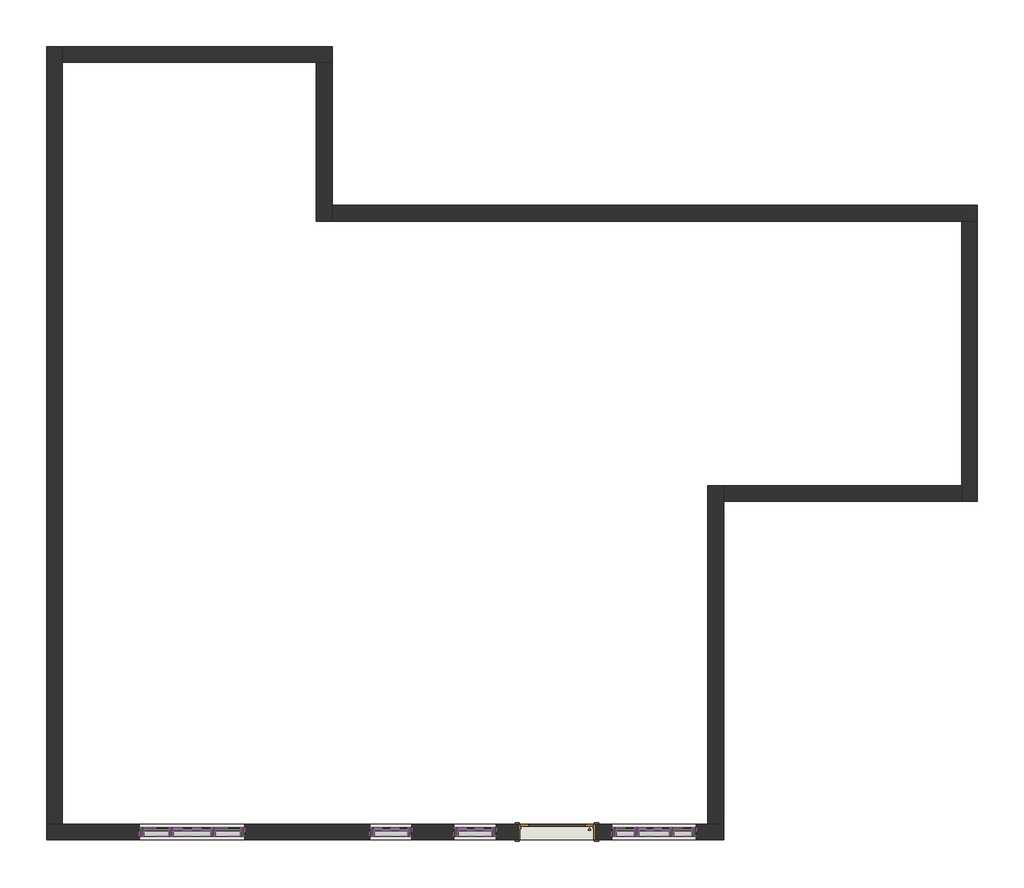
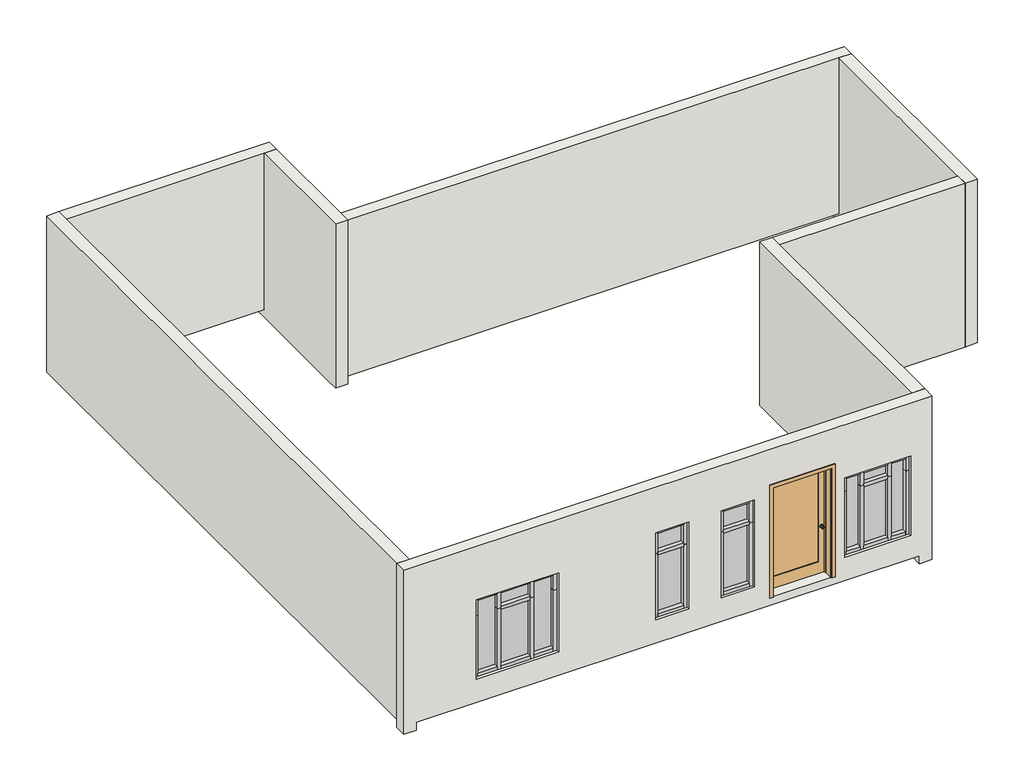
# One storey: 44 members, 12 plates, 8 walls, 1 door.
"""IFC4 building model written with IfcOpenShell, lengths in millimetres."""

from ifc_helpers import new_model, si_unit, frame, origin, place, context, project, spatial, polyline, outline, extrude, faceted_brep, transform, mapped, element, save
from components import door_0f538abb, member_86d06fe4, member_323df77c, member_71eb4692, member_843225dc, member_2d647432, member_0a1a1ade, member_a980948f, member_83167d3d, member_15823cb3, member_ca359333, member_ffcd2ccf, member_3c3dc66a, member_4adcbd6e, member_bc7dbe04, member_a1da5be3, member_718fe5d9, member_75d1e245, system_panel_glazed_030ff9b4, system_panel_glazed_82984963, system_panel_glazed_5eb04348, system_panel_glazed_6fd79a86, system_panel_glazed_80b64450, system_panel_glazed_1627a9b9, system_panel_glazed_6ade1748, system_panel_glazed_28683af0, system_panel_glazed_ad29da2a, system_panel_glazed_c196d27b

model = new_model("IFC4")

# Units and contexts
model_context = context("Model", 3, world=origin())
ifc_project = project(units=[si_unit("LENGTHUNIT", "METRE", prefix="MILLI")], contexts=[model_context])

# Site, building, storey
site = spatial("IfcSite", under=ifc_project)
building = spatial("IfcBuilding", under=site)
storey = spatial("IfcBuildingStorey", under=building, Elevation=3810.0)

# Door
placement = place(None, origin())
door_shape = door_0f538abb(model_context)
element("IfcDoor", 1, ObjectType="Door-Interior-Single-1_Panel-Wood : 3'6\" x 7' DOOR", at=placement, inside=storey, context=model_context, shape_type="MappedRepresentation", body=[
    mapped(door_shape, transform((3092.6850465, -1361.1591804, 4114.8), x_axis=(-1.0, 0.0, 0.0), y_axis=(0.0, -1.0, 0.0), z_axis=(0.0, 0.0, 1.0))),
])

# Members
member_shape = member_86d06fe4(model_context)
element("IfcMember", 2, ObjectType="Rectangular Mullion : 2.5\" x 5\" rectangular", at=placement, inside=storey, context=model_context, shape_type="MappedRepresentation", body=[
    mapped(member_shape, transform((940.0350465, -1364.3341804, 6121.4), x_axis=(0.0, 0.0, 1.0), y_axis=(0.0, -1.0, 0.0), z_axis=(1.0, 0.0, 0.0))),
])
element("IfcMember", 3, ObjectType="Rectangular Mullion : 2.5\" x 5\" rectangular", at=placement, inside=storey, context=model_context, shape_type="MappedRepresentation", body=[
    mapped(member_shape, transform((457.4350465, -1364.3341804, 4419.6), x_axis=(0.0, 0.0, -1.0), y_axis=(0.0, -1.0, 0.0), z_axis=(-1.0, 0.0, 0.0))),
])
member_2_shape = member_323df77c(model_context)
element("IfcMember", 4, ObjectType="Rectangular Mullion : 2.5\" x 5\" rectangular", at=placement, inside=storey, context=model_context, shape_type="MappedRepresentation", body=[
    mapped(member_2_shape, transform((940.0350465, -1364.3341804, 5664.2), x_axis=(0.0, 0.0, 1.0), y_axis=(0.0, -1.0, 0.0), z_axis=(1.0, 0.0, 0.0))),
])
member_3_shape = member_71eb4692(model_context)
element("IfcMember", 5, ObjectType="Rectangular Mullion : 2.5\" x 5\" rectangular", at=placement, inside=storey, context=model_context, shape_type="MappedRepresentation", body=[
    mapped(member_3_shape, transform((1003.5350465, -1364.3341804, 4419.6), x_axis=(1.0, 0.0, 0.0), y_axis=(0.0, -1.0, 0.0), z_axis=(0.0, 0.0, -1.0))),
])
element("IfcMember", 6, ObjectType="Rectangular Mullion : 2.5\" x 5\" rectangular", at=placement, inside=storey, context=model_context, shape_type="MappedRepresentation", body=[
    mapped(member_3_shape, transform((393.9350465, -1364.3341804, 5664.2), x_axis=(-1.0, 0.0, 0.0), y_axis=(0.0, -1.0, 0.0), z_axis=(0.0, 0.0, 1.0))),
])
element("IfcMember", 7, ObjectType="Rectangular Mullion : 2.5\" x 5\" rectangular", at=placement, inside=storey, context=model_context, shape_type="MappedRepresentation", body=[
    mapped(member_shape, transform((1670.2850465, -1364.3341804, 6121.4), x_axis=(0.0, 0.0, 1.0), y_axis=(0.0, 1.0, 0.0), z_axis=(-1.0, 0.0, 0.0))),
])
element("IfcMember", 8, ObjectType="Rectangular Mullion : 2.5\" x 5\" rectangular", at=placement, inside=storey, context=model_context, shape_type="MappedRepresentation", body=[
    mapped(member_shape, transform((2152.8850465, -1364.3341804, 4419.6), x_axis=(0.0, 0.0, -1.0), y_axis=(0.0, 1.0, 0.0), z_axis=(1.0, 0.0, 0.0))),
])
element("IfcMember", 9, ObjectType="Rectangular Mullion : 2.5\" x 5\" rectangular", at=placement, inside=storey, context=model_context, shape_type="MappedRepresentation", body=[
    mapped(member_2_shape, transform((1670.2850465, -1364.3341804, 5664.2), x_axis=(0.0, 0.0, 1.0), y_axis=(0.0, 1.0, 0.0), z_axis=(-1.0, 0.0, 0.0))),
])
element("IfcMember", 10, ObjectType="Rectangular Mullion : 2.5\" x 5\" rectangular", at=placement, inside=storey, context=model_context, shape_type="MappedRepresentation", body=[
    mapped(member_3_shape, transform((1606.7850465, -1364.3341804, 4419.6), x_axis=(-1.0, 0.0, 0.0), y_axis=(0.0, 1.0, 0.0), z_axis=(0.0, 0.0, -1.0))),
])
element("IfcMember", 11, ObjectType="Rectangular Mullion : 2.5\" x 5\" rectangular", at=placement, inside=storey, context=model_context, shape_type="MappedRepresentation", body=[
    mapped(member_3_shape, transform((2216.3850465, -1364.3341804, 5664.2), x_axis=(1.0, 0.0, 0.0), y_axis=(0.0, 1.0, 0.0), z_axis=(0.0, 0.0, 1.0))),
])
member_4_shape = member_843225dc(model_context)
element("IfcMember", 12, ObjectType="Rectangular Mullion : 2.5\" x 5\" rectangular", at=placement, inside=storey, context=model_context, shape_type="MappedRepresentation", body=[
    mapped(member_4_shape, transform((-1466.6149535, -1364.3341804, 5969.0), x_axis=(0.0, 0.0, 1.0), y_axis=(0.0, -1.0, 0.0), z_axis=(1.0, 0.0, 0.0))),
])
element("IfcMember", 13, ObjectType="Rectangular Mullion : 2.5\" x 5\" rectangular", at=placement, inside=storey, context=model_context, shape_type="MappedRepresentation", body=[
    mapped(member_4_shape, transform((-2501.6649535, -1364.3341804, 5969.0), x_axis=(0.0, 0.0, 1.0), y_axis=(0.0, -1.0, 0.0), z_axis=(1.0, 0.0, 0.0))),
])
element("IfcMember", 14, ObjectType="Rectangular Mullion : 2.5\" x 5\" rectangular", at=placement, inside=storey, context=model_context, shape_type="MappedRepresentation", body=[
    mapped(member_4_shape, transform((-2863.6149535, -1364.3341804, 4419.6), x_axis=(0.0, 0.0, -1.0), y_axis=(0.0, -1.0, 0.0), z_axis=(-1.0, 0.0, 0.0))),
])
element("IfcMember", 15, ObjectType="Rectangular Mullion : 2.5\" x 5\" rectangular", at=placement, inside=storey, context=model_context, shape_type="MappedRepresentation", body=[
    mapped(member_4_shape, transform((-1828.5649535, -1364.3341804, 4419.6), x_axis=(0.0, 0.0, -1.0), y_axis=(0.0, -1.0, 0.0), z_axis=(-1.0, 0.0, 0.0))),
])
member_5_shape = member_2d647432(model_context)
element("IfcMember", 16, ObjectType="Rectangular Mullion : 2.5\" x 5\" rectangular", at=placement, inside=storey, context=model_context, shape_type="MappedRepresentation", body=[
    mapped(member_5_shape, transform((-2469.9149535, -1364.3341804, 4419.6), x_axis=(1.0, 0.0, 0.0), y_axis=(0.0, -1.0, 0.0), z_axis=(0.0, 0.0, -1.0))),
])
element("IfcMember", 17, ObjectType="Rectangular Mullion : 2.5\" x 5\" rectangular", at=placement, inside=storey, context=model_context, shape_type="MappedRepresentation", body=[
    mapped(member_5_shape, transform((-1860.3149535, -1364.3341804, 4419.6), x_axis=(1.0, 0.0, 0.0), y_axis=(0.0, -1.0, 0.0), z_axis=(0.0, 0.0, -1.0))),
])
member_6_shape = member_0a1a1ade(model_context)
element("IfcMember", 18, ObjectType="Rectangular Mullion : 2.5\" x 5\" rectangular", at=placement, inside=storey, context=model_context, shape_type="MappedRepresentation", body=[
    mapped(member_6_shape, transform((-1892.0649535, -1364.3341804, 5613.4), x_axis=(0.0, 0.0, 1.0), y_axis=(0.0, -1.0, 0.0), z_axis=(1.0, 0.0, 0.0))),
])
member_7_shape = member_a980948f(model_context)
element("IfcMember", 19, ObjectType="Rectangular Mullion : 2.5\" x 5\" rectangular", at=placement, inside=storey, context=model_context, shape_type="MappedRepresentation", body=[
    mapped(member_7_shape, transform((-2438.1649535, -1364.3341804, 4419.6), x_axis=(0.0, 0.0, -1.0), y_axis=(0.0, -1.0, 0.0), z_axis=(-1.0, 0.0, 0.0))),
])
element("IfcMember", 20, ObjectType="Rectangular Mullion : 2.5\" x 5\" rectangular", at=placement, inside=storey, context=model_context, shape_type="MappedRepresentation", body=[
    mapped(member_7_shape, transform((-1892.0649535, -1364.3341804, 5969.0), x_axis=(0.0, 0.0, 1.0), y_axis=(0.0, -1.0, 0.0), z_axis=(1.0, 0.0, 0.0))),
])
member_8_shape = member_83167d3d(model_context)
element("IfcMember", 21, ObjectType="Rectangular Mullion : 2.5\" x 5\" rectangular", at=placement, inside=storey, context=model_context, shape_type="MappedRepresentation", body=[
    mapped(member_8_shape, transform((-1403.1149535, -1364.3341804, 4419.6), x_axis=(1.0, 0.0, 0.0), y_axis=(0.0, -1.0, 0.0), z_axis=(0.0, 0.0, -1.0))),
])
element("IfcMember", 22, ObjectType="Rectangular Mullion : 2.5\" x 5\" rectangular", at=placement, inside=storey, context=model_context, shape_type="MappedRepresentation", body=[
    mapped(member_8_shape, transform((-2927.1149535, -1364.3341804, 5613.4), x_axis=(-1.0, 0.0, 0.0), y_axis=(0.0, -1.0, 0.0), z_axis=(0.0, 0.0, 1.0))),
])
member_9_shape = member_15823cb3(model_context)
element("IfcMember", 23, ObjectType="Rectangular Mullion : 2.5\" x 5\" rectangular", at=placement, inside=storey, context=model_context, shape_type="MappedRepresentation", body=[
    mapped(member_9_shape, transform((393.9350465, -1364.3341804, 6121.4), x_axis=(-1.0, 0.0, 0.0), y_axis=(0.0, -1.0, 0.0), z_axis=(0.0, 0.0, 1.0))),
])
element("IfcMember", 24, ObjectType="Rectangular Mullion : 2.5\" x 5\" rectangular", at=placement, inside=storey, context=model_context, shape_type="MappedRepresentation", body=[
    mapped(member_9_shape, transform((1003.5350465, -1364.3341804, 5664.2), x_axis=(1.0, 0.0, 0.0), y_axis=(0.0, -1.0, 0.0), z_axis=(0.0, 0.0, -1.0))),
])
element("IfcMember", 25, ObjectType="Rectangular Mullion : 2.5\" x 5\" rectangular", at=placement, inside=storey, context=model_context, shape_type="MappedRepresentation", body=[
    mapped(member_9_shape, transform((2216.3850465, -1364.3341804, 6121.4), x_axis=(1.0, 0.0, 0.0), y_axis=(0.0, 1.0, 0.0), z_axis=(0.0, 0.0, 1.0))),
])
element("IfcMember", 26, ObjectType="Rectangular Mullion : 2.5\" x 5\" rectangular", at=placement, inside=storey, context=model_context, shape_type="MappedRepresentation", body=[
    mapped(member_9_shape, transform((1606.7850465, -1364.3341804, 5664.2), x_axis=(-1.0, 0.0, 0.0), y_axis=(0.0, 1.0, 0.0), z_axis=(0.0, 0.0, -1.0))),
])
member_10_shape = member_ca359333(model_context)
element("IfcMember", 27, ObjectType="Rectangular Mullion : 2.5\" x 5\" rectangular", at=placement, inside=storey, context=model_context, shape_type="MappedRepresentation", body=[
    mapped(member_10_shape, transform((-2469.9149535, -1364.3341804, 5613.4), x_axis=(1.0, 0.0, 0.0), y_axis=(0.0, -1.0, 0.0), z_axis=(0.0, 0.0, -1.0))),
])
element("IfcMember", 28, ObjectType="Rectangular Mullion : 2.5\" x 5\" rectangular", at=placement, inside=storey, context=model_context, shape_type="MappedRepresentation", body=[
    mapped(member_10_shape, transform((-1860.3149535, -1364.3341804, 5613.4), x_axis=(1.0, 0.0, 0.0), y_axis=(0.0, -1.0, 0.0), z_axis=(0.0, 0.0, -1.0))),
])
member_11_shape = member_ffcd2ccf(model_context)
element("IfcMember", 29, ObjectType="Rectangular Mullion : 2.5\" x 5\" rectangular", at=placement, inside=storey, context=model_context, shape_type="MappedRepresentation", body=[
    mapped(member_11_shape, transform((-2927.1149535, -1364.3341804, 5969.0), x_axis=(-1.0, 0.0, 0.0), y_axis=(0.0, -1.0, 0.0), z_axis=(0.0, 0.0, 1.0))),
])
element("IfcMember", 30, ObjectType="Rectangular Mullion : 2.5\" x 5\" rectangular", at=placement, inside=storey, context=model_context, shape_type="MappedRepresentation", body=[
    mapped(member_11_shape, transform((-1403.1149535, -1364.3341804, 5613.4), x_axis=(1.0, 0.0, 0.0), y_axis=(0.0, -1.0, 0.0), z_axis=(0.0, 0.0, -1.0))),
])
member_12_shape = member_3c3dc66a(model_context)
element("IfcMember", 31, ObjectType="Rectangular Mullion : 2.5\" x 5\" rectangular", at=placement, inside=storey, context=model_context, shape_type="MappedRepresentation", body=[
    mapped(member_12_shape, transform((3880.0850465, -1364.3341804, 5969.0), x_axis=(-1.0, 0.0, 0.0), y_axis=(0.0, -1.0, 0.0), z_axis=(0.0, 0.0, 1.0))),
])
element("IfcMember", 32, ObjectType="Rectangular Mullion : 2.5\" x 5\" rectangular", at=placement, inside=storey, context=model_context, shape_type="MappedRepresentation", body=[
    mapped(member_3_shape, transform((5099.2850465, -1364.3341804, 4419.6), x_axis=(1.0, 0.0, 0.0), y_axis=(0.0, -1.0, 0.0), z_axis=(0.0, 0.0, -1.0))),
])
element("IfcMember", 33, ObjectType="Rectangular Mullion : 2.5\" x 5\" rectangular", at=placement, inside=storey, context=model_context, shape_type="MappedRepresentation", body=[
    mapped(member_12_shape, transform((5099.2850465, -1364.3341804, 5664.2), x_axis=(1.0, 0.0, 0.0), y_axis=(0.0, -1.0, 0.0), z_axis=(0.0, 0.0, -1.0))),
])
element("IfcMember", 34, ObjectType="Rectangular Mullion : 2.5\" x 5\" rectangular", at=placement, inside=storey, context=model_context, shape_type="MappedRepresentation", body=[
    mapped(member_3_shape, transform((3880.0850465, -1364.3341804, 5664.2), x_axis=(-1.0, 0.0, 0.0), y_axis=(0.0, -1.0, 0.0), z_axis=(0.0, 0.0, 1.0))),
])
member_13_shape = member_4adcbd6e(model_context)
element("IfcMember", 35, ObjectType="Rectangular Mullion : 2.5\" x 5\" rectangular", at=placement, inside=storey, context=model_context, shape_type="MappedRepresentation", body=[
    mapped(member_13_shape, transform((5035.7850465, -1364.3341804, 5969.0), x_axis=(0.0, 0.0, 1.0), y_axis=(0.0, -1.0, 0.0), z_axis=(1.0, 0.0, 0.0))),
])
element("IfcMember", 36, ObjectType="Rectangular Mullion : 2.5\" x 5\" rectangular", at=placement, inside=storey, context=model_context, shape_type="MappedRepresentation", body=[
    mapped(member_13_shape, transform((4203.9350465, -1364.3341804, 5969.0), x_axis=(0.0, 0.0, 1.0), y_axis=(0.0, -1.0, 0.0), z_axis=(1.0, 0.0, 0.0))),
])
element("IfcMember", 37, ObjectType="Rectangular Mullion : 2.5\" x 5\" rectangular", at=placement, inside=storey, context=model_context, shape_type="MappedRepresentation", body=[
    mapped(member_13_shape, transform((3943.5850465, -1364.3341804, 4419.6), x_axis=(0.0, 0.0, -1.0), y_axis=(0.0, -1.0, 0.0), z_axis=(-1.0, 0.0, 0.0))),
])
element("IfcMember", 38, ObjectType="Rectangular Mullion : 2.5\" x 5\" rectangular", at=placement, inside=storey, context=model_context, shape_type="MappedRepresentation", body=[
    mapped(member_13_shape, transform((4775.4350465, -1364.3341804, 4419.6), x_axis=(0.0, 0.0, -1.0), y_axis=(0.0, -1.0, 0.0), z_axis=(-1.0, 0.0, 0.0))),
])
member_14_shape = member_bc7dbe04(model_context)
element("IfcMember", 39, ObjectType="Rectangular Mullion : 2.5\" x 5\" rectangular", at=placement, inside=storey, context=model_context, shape_type="MappedRepresentation", body=[
    mapped(member_14_shape, transform((4267.4350465, -1364.3341804, 4419.6), x_axis=(0.0, 0.0, -1.0), y_axis=(0.0, -1.0, 0.0), z_axis=(-1.0, 0.0, 0.0))),
])
element("IfcMember", 40, ObjectType="Rectangular Mullion : 2.5\" x 5\" rectangular", at=placement, inside=storey, context=model_context, shape_type="MappedRepresentation", body=[
    mapped(member_14_shape, transform((4711.9350465, -1364.3341804, 5969.0), x_axis=(0.0, 0.0, 1.0), y_axis=(0.0, -1.0, 0.0), z_axis=(1.0, 0.0, 0.0))),
])
member_15_shape = member_a1da5be3(model_context)
element("IfcMember", 41, ObjectType="Rectangular Mullion : 2.5\" x 5\" rectangular", at=placement, inside=storey, context=model_context, shape_type="MappedRepresentation", body=[
    mapped(member_15_shape, transform((4235.6850465, -1364.3341804, 4419.6), x_axis=(1.0, 0.0, 0.0), y_axis=(0.0, -1.0, 0.0), z_axis=(0.0, 0.0, -1.0))),
])
element("IfcMember", 42, ObjectType="Rectangular Mullion : 2.5\" x 5\" rectangular", at=placement, inside=storey, context=model_context, shape_type="MappedRepresentation", body=[
    mapped(member_15_shape, transform((4743.6850465, -1364.3341804, 4419.6), x_axis=(1.0, 0.0, 0.0), y_axis=(0.0, -1.0, 0.0), z_axis=(0.0, 0.0, -1.0))),
])
member_16_shape = member_718fe5d9(model_context)
element("IfcMember", 43, ObjectType="Rectangular Mullion : 2.5\" x 5\" rectangular", at=placement, inside=storey, context=model_context, shape_type="MappedRepresentation", body=[
    mapped(member_16_shape, transform((4711.9350465, -1364.3341804, 5664.2), x_axis=(0.0, 0.0, 1.0), y_axis=(0.0, -1.0, 0.0), z_axis=(1.0, 0.0, 0.0))),
])
member_17_shape = member_75d1e245(model_context)
element("IfcMember", 44, ObjectType="Rectangular Mullion : 2.5\" x 5\" rectangular", at=placement, inside=storey, context=model_context, shape_type="MappedRepresentation", body=[
    mapped(member_17_shape, transform((4235.6850465, -1364.3341804, 5664.2), x_axis=(1.0, 0.0, 0.0), y_axis=(0.0, -1.0, 0.0), z_axis=(0.0, 0.0, -1.0))),
])
element("IfcMember", 45, ObjectType="Rectangular Mullion : 2.5\" x 5\" rectangular", at=placement, inside=storey, context=model_context, shape_type="MappedRepresentation", body=[
    mapped(member_17_shape, transform((4743.6850465, -1364.3341804, 5664.2), x_axis=(1.0, 0.0, 0.0), y_axis=(0.0, -1.0, 0.0), z_axis=(0.0, 0.0, -1.0))),
])

# Plates
system_panel_glazed_shape = system_panel_glazed_030ff9b4(model_context)
element("IfcPlate", 46, ObjectType="System Panel : Glazed", at=placement, inside=storey, context=model_context, shape_type="MappedRepresentation", body=[
    mapped(system_panel_glazed_shape, transform((698.7350465, -1364.3341804, 4483.1), x_axis=(1.0, 0.0, 0.0), y_axis=(0.0, 1.0, 0.0), z_axis=(0.0, 0.0, 1.0))),
])
system_panel_glazed_2_shape = system_panel_glazed_82984963(model_context)
element("IfcPlate", 47, ObjectType="System Panel : Glazed", at=placement, inside=storey, context=model_context, shape_type="MappedRepresentation", body=[
    mapped(system_panel_glazed_2_shape, transform((1911.5850465, -1364.3341804, 4483.1), x_axis=(-1.0, 0.0, 0.0), y_axis=(0.0, -1.0, 0.0), z_axis=(0.0, 0.0, 1.0))),
])
system_panel_glazed_3_shape = system_panel_glazed_5eb04348(model_context)
element("IfcPlate", 48, ObjectType="System Panel : Glazed", at=placement, inside=storey, context=model_context, shape_type="MappedRepresentation", body=[
    mapped(system_panel_glazed_3_shape, transform((-2165.1149535, -1364.3341804, 4483.1), x_axis=(1.0, 0.0, 0.0), y_axis=(0.0, 1.0, 0.0), z_axis=(0.0, 0.0, 1.0))),
])
system_panel_glazed_4_shape = system_panel_glazed_6fd79a86(model_context)
element("IfcPlate", 49, ObjectType="System Panel : Glazed", at=placement, inside=storey, context=model_context, shape_type="MappedRepresentation", body=[
    mapped(system_panel_glazed_4_shape, transform((698.7350465, -1364.3341804, 5695.95), x_axis=(1.0, 0.0, 0.0), y_axis=(0.0, 1.0, 0.0), z_axis=(0.0, 0.0, 1.0))),
])
system_panel_glazed_5_shape = system_panel_glazed_80b64450(model_context)
element("IfcPlate", 50, ObjectType="System Panel : Glazed", at=placement, inside=storey, context=model_context, shape_type="MappedRepresentation", body=[
    mapped(system_panel_glazed_5_shape, transform((1911.5850465, -1364.3341804, 5695.95), x_axis=(-1.0, 0.0, 0.0), y_axis=(0.0, -1.0, 0.0), z_axis=(0.0, 0.0, 1.0))),
])
system_panel_glazed_6_shape = system_panel_glazed_1627a9b9(model_context)
element("IfcPlate", 51, ObjectType="System Panel : Glazed", at=placement, inside=storey, context=model_context, shape_type="MappedRepresentation", body=[
    mapped(system_panel_glazed_6_shape, transform((-2682.6399535, -1364.3341804, 4483.1), x_axis=(1.0, 0.0, 0.0), y_axis=(0.0, 1.0, 0.0), z_axis=(0.0, 0.0, 1.0))),
])
element("IfcPlate", 52, ObjectType="System Panel : Glazed", at=placement, inside=storey, context=model_context, shape_type="MappedRepresentation", body=[
    mapped(system_panel_glazed_6_shape, transform((-1647.5899535, -1364.3341804, 4483.1), x_axis=(1.0, 0.0, 0.0), y_axis=(0.0, 1.0, 0.0), z_axis=(0.0, 0.0, 1.0))),
])
system_panel_glazed_7_shape = system_panel_glazed_6ade1748(model_context)
element("IfcPlate", 53, ObjectType="System Panel : Glazed", at=placement, inside=storey, context=model_context, shape_type="MappedRepresentation", body=[
    mapped(system_panel_glazed_7_shape, transform((-2165.1149535, -1364.3341804, 5645.15), x_axis=(1.0, 0.0, 0.0), y_axis=(0.0, 1.0, 0.0), z_axis=(0.0, 0.0, 1.0))),
])
system_panel_glazed_8_shape = system_panel_glazed_28683af0(model_context)
element("IfcPlate", 54, ObjectType="System Panel : Glazed", at=placement, inside=storey, context=model_context, shape_type="MappedRepresentation", body=[
    mapped(system_panel_glazed_8_shape, transform((4073.7600465, -1364.3341804, 4483.1), x_axis=(1.0, 0.0, 0.0), y_axis=(0.0, 1.0, 0.0), z_axis=(0.0, 0.0, 1.0))),
])
element("IfcPlate", 55, ObjectType="System Panel : Glazed", at=placement, inside=storey, context=model_context, shape_type="MappedRepresentation", body=[
    mapped(system_panel_glazed_8_shape, transform((4905.6100465, -1364.3341804, 4483.1), x_axis=(1.0, 0.0, 0.0), y_axis=(0.0, 1.0, 0.0), z_axis=(0.0, 0.0, 1.0))),
])
system_panel_glazed_9_shape = system_panel_glazed_ad29da2a(model_context)
element("IfcPlate", 56, ObjectType="System Panel : Glazed", at=placement, inside=storey, context=model_context, shape_type="MappedRepresentation", body=[
    mapped(system_panel_glazed_9_shape, transform((4489.6850465, -1364.3341804, 4483.1), x_axis=(1.0, 0.0, 0.0), y_axis=(0.0, 1.0, 0.0), z_axis=(0.0, 0.0, 1.0))),
])
system_panel_glazed_10_shape = system_panel_glazed_c196d27b(model_context)
element("IfcPlate", 57, ObjectType="System Panel : Glazed", at=placement, inside=storey, context=model_context, shape_type="MappedRepresentation", body=[
    mapped(system_panel_glazed_10_shape, transform((4489.6850465, -1364.3341804, 5695.95), x_axis=(1.0, 0.0, 0.0), y_axis=(0.0, 1.0, 0.0), z_axis=(0.0, 0.0, 1.0))),
])

# Walls
element("IfcWall", 58, ObjectType="9\" wall", at=placement, inside=storey, context=model_context, shape_type="Brep", body=[
    faceted_brep([(-4260.6149535, 9951.3658196, 3962.4), (-4260.6149535, 9722.7658196, 3962.4), (-4260.6149535, -1250.0341804, 3962.4), (-4260.6149535, -1250.0341804, 7010.4), (-4260.6149535, 9951.3658196, 7010.4), (-4032.0149535, 9951.3658196, 3962.4), (-4032.0149535, 9951.3658196, 7010.4), (-4032.0149535, 9722.7658196, 7010.4), (-4032.0149535, -1250.0341804, 7010.4), (-4032.0149535, -1250.0341804, 3962.4), (-4032.0149535, 9722.7658196, 3962.4)], [[[0, 1, 2, 3, 4]], [[5, 6, 7, 8, 9, 10]], [[2, 1, 0, 5, 10, 9]], [[4, 3, 8, 7, 6]], [[0, 4, 6, 5]], [[3, 2, 9, 8]]]),
])
element("IfcWall", 59, ObjectType="9\" wall", at=placement, inside=storey, context=model_context, shape_type="Brep", body=[
    faceted_brep([(-4032.0149535, 9722.7658196, 3962.4), (-374.4149535, 9722.7658196, 3962.4), (-145.8149535, 9722.7658196, 3962.4), (-145.8149535, 9722.7658196, 7010.4), (-374.4149535, 9722.7658196, 7010.4), (-4032.0149535, 9722.7658196, 7010.4), (-4032.0149535, 9951.3658196, 3962.4), (-4032.0149535, 9951.3658196, 7010.4), (-145.8149535, 9951.3658196, 7010.4), (-145.8149535, 9951.3658196, 3962.4), (-374.4149535, 9951.3658196, 3962.4)], [[[0, 1, 2, 3, 4, 5]], [[6, 7, 8, 9, 10]], [[2, 1, 0, 6, 10, 9]], [[5, 4, 3, 8, 7]], [[0, 5, 7, 6]], [[3, 2, 9, 8]]]),
])
element("IfcWall", 60, ObjectType="9\" wall", at=placement, inside=storey, context=model_context, shape_type="Brep", body=[
    faceted_brep([(-374.4149535, 9951.3658196, 3810.0), (-374.4149535, 9722.7658196, 3810.0), (-374.4149535, 7665.3658196, 3810.0), (-374.4149535, 7436.7658196, 3810.0), (-374.4149535, 7436.7658196, 7010.4), (-374.4149535, 9722.7658196, 7010.4), (-374.4149535, 9722.7658196, 3962.4), (-374.4149535, 9951.3658196, 3962.4), (-145.8149535, 9951.3658196, 3810.0), (-145.8149535, 9951.3658196, 3962.4), (-145.8149535, 9722.7658196, 3962.4), (-145.8149535, 9722.7658196, 7010.4), (-145.8149535, 7665.3658196, 7010.4), (-145.8149535, 7436.7658196, 7010.4), (-145.8149535, 7436.7658196, 3962.4), (-145.8149535, 7436.7658196, 3810.0), (-145.8149535, 7665.3658196, 3810.0), (-145.8149535, 9722.7658196, 3810.0)], [[[0, 1, 2, 3, 4, 5, 6, 7]], [[8, 9, 10, 11, 12, 13, 14, 15, 16, 17]], [[3, 2, 1, 0, 8, 17, 16, 15]], [[5, 4, 13, 12, 11]], [[3, 15, 14, 13, 4]], [[6, 10, 9, 7]], [[0, 7, 9, 8]], [[6, 5, 11, 10]]]),
])
element("IfcWall", 61, ObjectType="9\" wall", at=placement, inside=storey, context=model_context, shape_type="Brep", body=[
    faceted_brep([(-145.8149535, 7436.7658196, 3962.4), (8921.9850465, 7436.7658196, 3962.4), (9150.5850465, 7436.7658196, 3962.4), (9150.5850465, 7436.7658196, 7010.4), (8921.9850465, 7436.7658196, 7010.4), (-145.8149535, 7436.7658196, 7010.4), (-145.8149535, 7665.3658196, 3962.4), (-145.8149535, 7665.3658196, 7010.4), (9150.5850465, 7665.3658196, 7010.4), (9150.5850465, 7665.3658196, 3962.4), (8921.9850465, 7665.3658196, 3962.4)], [[[0, 1, 2, 3, 4, 5]], [[6, 7, 8, 9, 10]], [[2, 1, 0, 6, 10, 9]], [[5, 4, 3, 8, 7]], [[0, 5, 7, 6]], [[3, 2, 9, 8]]]),
])
element("IfcWall", 62, ObjectType="9\" wall", at=placement, inside=storey, context=model_context, shape_type="Brep", body=[
    faceted_brep([(8921.9850465, 7665.3658196, 3810.0), (8921.9850465, 3626.7658196, 3810.0), (8921.9850465, 3398.1658196, 3810.0), (8921.9850465, 3398.1658196, 3962.4), (8921.9850465, 3398.1658196, 7010.4), (8921.9850465, 3626.7658196, 7010.4), (8921.9850465, 7436.7658196, 7010.4), (8921.9850465, 7436.7658196, 3962.4), (8921.9850465, 7665.3658196, 3962.4), (9150.5850465, 7665.3658196, 3810.0), (9150.5850465, 7665.3658196, 3962.4), (9150.5850465, 7436.7658196, 3962.4), (9150.5850465, 7436.7658196, 7010.4), (9150.5850465, 3398.1658196, 7010.4), (9150.5850465, 3398.1658196, 3810.0), (9150.5850465, 3626.7658196, 3810.0)], [[[0, 1, 2, 3, 4, 5, 6, 7, 8]], [[9, 10, 11, 12, 13, 14, 15]], [[2, 1, 0, 9, 15, 14]], [[6, 5, 4, 13, 12]], [[2, 14, 13, 4, 3]], [[7, 11, 10, 8]], [[0, 8, 10, 9]], [[7, 6, 12, 11]]]),
])
element("IfcWall", 63, ObjectType="9\" wall", at=placement, inside=storey, context=model_context, shape_type="Brep", body=[
    faceted_brep([(-4260.6149535, -1250.0341804, 7010.4), (-4032.0149535, -1250.0341804, 7010.4), (5264.3850465, -1250.0341804, 7010.4), (5492.9850465, -1250.0341804, 7010.4), (5492.9850465, -1250.0341804, 3962.4), (5492.9850465, -1250.0341804, 3810.0), (5264.3850465, -1250.0341804, 3810.0), (5264.3850465, -1250.0341804, 3962.4), (-4032.0149535, -1250.0341804, 3962.4), (-4032.0149535, -1250.0341804, 3810.0), (-4260.6149535, -1250.0341804, 3810.0), (-4260.6149535, -1250.0341804, 3962.4), (2533.8850465, -1250.0341804, 6273.8), (2533.8850465, -1250.0341804, 4114.8), (3651.4850465, -1250.0341804, 4114.8), (3651.4850465, -1250.0341804, 6273.8), (393.9350465, -1250.0341804, 6121.4), (393.9350465, -1250.0341804, 4419.6), (1003.5350465, -1250.0341804, 4419.6), (1003.5350465, -1250.0341804, 6121.4), (2216.3850465, -1250.0341804, 4419.6), (2216.3850465, -1250.0341804, 6121.4), (1606.7850465, -1250.0341804, 6121.4), (1606.7850465, -1250.0341804, 4419.6), (3880.0850465, -1250.0341804, 5969.0), (3880.0850465, -1250.0341804, 4419.6), (5099.2850465, -1250.0341804, 4419.6), (5099.2850465, -1250.0341804, 5969.0), (-2927.1149535, -1250.0341804, 5969.0), (-2927.1149535, -1250.0341804, 4419.6), (-1403.1149535, -1250.0341804, 4419.6), (-1403.1149535, -1250.0341804, 5969.0), (5492.9850465, -1478.6341804, 7010.4), (-4260.6149535, -1478.6341804, 7010.4), (-4260.6149535, -1478.6341804, 3810.0), (-4032.0149535, -1478.6341804, 3810.0), (-4032.0149535, -1478.6341804, 3962.4), (5264.3850465, -1478.6341804, 3962.4), (5264.3850465, -1478.6341804, 3810.0), (5492.9850465, -1478.6341804, 3810.0), (2533.8850465, -1478.6341804, 4114.8), (2533.8850465, -1478.6341804, 6273.8), (3651.4850465, -1478.6341804, 6273.8), (3651.4850465, -1478.6341804, 4114.8), (393.9350465, -1478.6341804, 4419.6), (393.9350465, -1478.6341804, 6121.4), (1003.5350465, -1478.6341804, 6121.4), (1003.5350465, -1478.6341804, 4419.6), (2216.3850465, -1478.6341804, 6121.4), (2216.3850465, -1478.6341804, 4419.6), (1606.7850465, -1478.6341804, 4419.6), (1606.7850465, -1478.6341804, 6121.4), (3880.0850465, -1478.6341804, 4419.6), (3880.0850465, -1478.6341804, 5969.0), (5099.2850465, -1478.6341804, 5969.0), (5099.2850465, -1478.6341804, 4419.6), (-2927.1149535, -1478.6341804, 4419.6), (-2927.1149535, -1478.6341804, 5969.0), (-1403.1149535, -1478.6341804, 5969.0), (-1403.1149535, -1478.6341804, 4419.6)], [[[0, 1, 2, 3, 4, 5, 6, 7, 8, 9, 10, 11], [12, 13, 14, 15], [16, 17, 18, 19], [20, 21, 22, 23], [24, 25, 26, 27], [28, 29, 30, 31]], [[32, 33, 34, 35, 36, 37, 38, 39], [40, 41, 42, 43], [44, 45, 46, 47], [48, 49, 50, 51], [52, 53, 54, 55], [56, 57, 58, 59]], [[34, 10, 9, 35]], [[5, 39, 38, 6]], [[3, 2, 1, 0, 33, 32]], [[40, 13, 12, 41]], [[41, 12, 15, 42]], [[42, 15, 14, 43]], [[13, 40, 43, 14]], [[44, 17, 16, 45]], [[45, 16, 19, 46]], [[46, 19, 18, 47]], [[17, 44, 47, 18]], [[20, 49, 48, 21]], [[21, 48, 51, 22]], [[22, 51, 50, 23]], [[49, 20, 23, 50]], [[8, 36, 35, 9]], [[36, 8, 7, 37]], [[37, 7, 6, 38]], [[3, 32, 39, 5, 4]], [[10, 34, 33, 0, 11]], [[52, 25, 24, 53]], [[53, 24, 27, 54]], [[54, 27, 26, 55]], [[25, 52, 55, 26]], [[56, 29, 28, 57]], [[57, 28, 31, 58]], [[58, 31, 30, 59]], [[29, 56, 59, 30]]]),
])
element("IfcWall", 64, ObjectType="9\" wall", at=placement, inside=storey, context=model_context, shape_type="Brep", body=[
    faceted_brep([(5492.9850465, -1250.0341804, 7010.4), (5492.9850465, -1250.0341804, 3810.0), (5492.9850465, 3398.1658196, 3810.0), (5492.9850465, 3626.7658196, 3810.0), (5492.9850465, 3626.7658196, 7010.4), (5492.9850465, 3398.1658196, 7010.4), (5264.3850465, -1250.0341804, 3810.0), (5264.3850465, -1250.0341804, 7010.4), (5264.3850465, 3626.7658196, 7010.4), (5264.3850465, 3626.7658196, 3810.0)], [[[0, 1, 2, 3, 4, 5]], [[6, 7, 8, 9]], [[3, 2, 1, 6, 9]], [[0, 5, 4, 8, 7]], [[4, 3, 9, 8]], [[0, 7, 6, 1]]]),
])
element("IfcWall", 65, ObjectType="9\" wall", at=placement, inside=storey, context=model_context, shape_type="SweptSolid", body=[
    extrude(outline(polyline([(5492.9850465, 3626.7658196), (8921.9850465, 3626.7658196), (8921.9850465, 3398.1658196), (5492.9850465, 3398.1658196), (5492.9850465, 3626.7658196)])), frame((0.0, 0.0, 3810.0), z_axis=(0.0, 0.0, 1.0), x_axis=(1.0, 0.0, 0.0)), (0.0, 0.0, 1.0), 3200.4),
])

save(model, "model.ifc")

# Revit data of these elements
# Type "Door-Interior-Single-1_Panel-Wood : 3'6\" x 7' DOOR"
#   Type Mark = "9"
#   Assembly Code = "C1020300"
#   Analytic Construction = "Wooden"
#   Top Rail = 0' - 4 11/16"
#   Thickness = 0' - 1 3/8"
#   Thermal Resistance (R) = 2.5876 (h·ft²·°F)/BTU
#   Swing Angle [instance default] = 90.00°
#   Stiles = 0' - 4 3/4"
#   Rough Width = 3' - 8"
#   Rough Height = 7' - 1"
#   Height = 7' - 0"
#   Width = 3' - 6"
#   Heat Transfer Coefficient (U) = 0.3865 BTU/(h·ft²·°F)
#   Bottom Rail = 0' - 9 1/8"
#   Trim Material = DOOR 3'6" X 7'
#   Panel Material = DOOR 3'6" X 7'
#   Frame Material = DOOR 3'6" X 7'
#   Door Handle Material = Aluminum
#   Visual Light Transmittance = 0
#   Solar Heat Gain Coefficient = 0
#   Wall Closure = (empty or 0)
#   Function = (empty or 0)
# Type "Rectangular Mullion : 2.5\" x 5\" rectangular"
#   built-in parameter 1007304 = 0.416667 (stored number, unit not read)
#   built-in parameter 1007301 = 0.104167 (stored number, unit not read)
#   built-in parameter 1007300 = 0.104167 (stored number, unit not read)
# Type "System Panel : Glazed"
#   Construction Type Id = "GSP4R"
#   Analytic Construction = "1/8 in Pilkington single glazing"
#   Visual Light Transmittance = 0.9
#   Solar Heat Gain Coefficient = 0.86
#   Heat Transfer Coefficient (U) = 1.18115 BTU/(h·ft²·°F)
#   Define Thermal Properties by = 1
# Type "9\" wall"
#   Assembly Code = "B2010"
#   Layers, outside or top first: 0' - 9" no material (function 1)
# Element 1 (IfcDoor, "Door-Interior-Single-1_Panel-Wood : 3'6\" x 7' DOOR")
#   Swing Angle = 90.00°
#   Phase Created = New Construction
#   Materials on its faces: "DOOR 3'6\" X 7'", "Aluminum"
# Elements 2, 3, 4, 5, 6, 7, 8, 9, 10, 11, 12, 13, 14, 15, 16, 17, 18, 19, 20, 21, 22, 23, 24, 25, 26, 27, 28, 29, 30, 31, 32, 33, 34, 35, 36, 37, 38, 39, 40, 41, 42, 43, 44, 45 (IfcMember, "Rectangular Mullion : 2.5\" x 5\" rectangular")
#   Phase Created = New Construction
# Elements 46, 47, 48, 49, 50, 51, 52, 53, 54, 55, 56, 57 (IfcPlate, "System Panel : Glazed")
#   Phase Created = New Construction
#   Materials on its faces: "Glass"
# Elements 58, 59, 61 (IfcWall, "9\" wall")
#   built-in parameter 1001111 = 0' - 6"
#   Top Offset = 0' - 0"
#   Base Offset = 0' - 6"
#   wall height = 10' - 0"
#   Phase Created = New Construction
#   Top Constraint = 5 SLAB L
#   Materials on its faces: "Default Wall"
# Elements 60, 62, 63, 64, 65 (IfcWall, "9\" wall")
#   Top Offset = 0' - 0"
#   Base Offset = 0' - 0"
#   wall height = 10' - 6"
#   Phase Created = New Construction
#   Top Constraint = 5 SLAB L
#   Materials on its faces: "Default Wall"
# Materials
#   "DOOR 3'6\" X 7'": class "Generic", colour RGB 120 120 120, transparency 0, Cost = 0
#   "Aluminum": class "Metal", colour RGB 247 247 247, transparency 0, Description = "Aluminum 6061", Cost = 0
#   "Glass": class "Glass", colour RGB 0 128 192, transparency 0.75, Description = "Soda Lime Glass", Cost = 0
#   "Default Wall": colour RGB 128 128 128, transparency 0, Cost = 0
